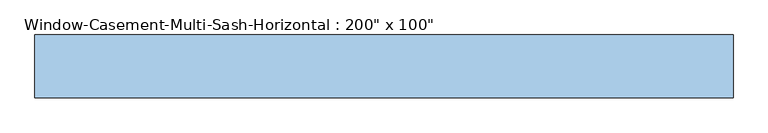
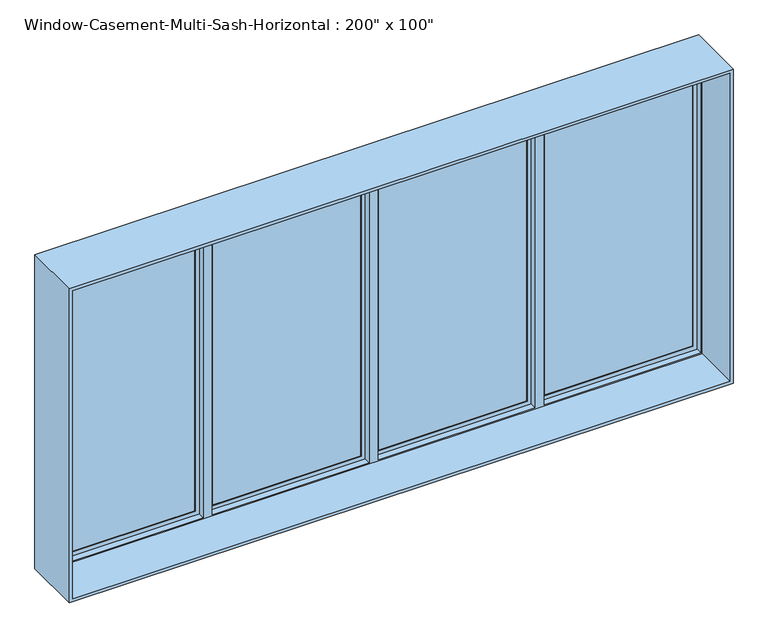
"""IFC4 building model written with IfcOpenShell, lengths in millimetres: window geometry."""

from ifc_helpers import new_model, si_unit, frame, origin, place, context, project, spatial, polyline, outline, extrude, faceted_brep, source, transform, mapped, element, save


def window_3db9eff8(model_context):
    return source(origin(), model_context, "Body", "SolidModel", [
        extrude(outline(polyline([(3429.0, 1295.4), (939.8, 1295.4), (939.8, 2514.6), (3429.0, 2514.6), (3429.0, 1295.4)]), holes=[polyline([(3387.1296875, 2472.7296875), (981.6703125, 2472.7296875), (981.6703125, 1337.2703125), (3387.1296875, 1337.2703125), (3387.1296875, 2472.7296875)])]), frame((0.0, 187.325, 0.0), z_axis=(0.0, 1.0, 0.0), x_axis=(0.0, 0.0, 1.0)), (0.0, 0.0, 1.0), 31.75),
        extrude(outline(polyline([(3429.0, -2514.6), (939.8, -2514.6), (939.8, -1295.4), (3429.0, -1295.4), (3429.0, -2514.6)]), holes=[polyline([(3387.1296875, -1337.2703125), (981.6703125, -1337.2703125), (981.6703125, -2472.7296875), (3387.1296875, -2472.7296875), (3387.1296875, -1337.2703125)])]), frame((0.0, 187.325, 0.0), z_axis=(0.0, 1.0, 0.0), x_axis=(0.0, 0.0, 1.0)), (0.0, 0.0, 1.0), 31.75),
        extrude(outline(polyline([(-1337.2703125, 212.725), (-1337.2703125, 206.375), (-2472.7296875, 206.375), (-2472.7296875, 212.725), (-1337.2703125, 212.725)])), frame((0.0, 0.0, 981.6703125), z_axis=(0.0, 0.0, 1.0), x_axis=(1.0, 0.0, 0.0)), (0.0, 0.0, 1.0), 2405.459375),
        extrude(outline(polyline([(-1337.2703125, 200.025), (-1337.2703125, 193.675), (-2472.7296875, 193.675), (-2472.7296875, 200.025), (-1337.2703125, 200.025)])), frame((0.0, 0.0, 981.6703125), z_axis=(0.0, 0.0, 1.0), x_axis=(1.0, 0.0, 0.0)), (0.0, 0.0, 1.0), 2405.459375),
        extrude(outline(polyline([(2472.7296875, 212.725), (2472.7296875, 206.375), (1337.2703125, 206.375), (1337.2703125, 212.725), (2472.7296875, 212.725)])), frame((0.0, 0.0, 981.6703125), z_axis=(0.0, 0.0, 1.0), x_axis=(1.0, 0.0, 0.0)), (0.0, 0.0, 1.0), 2405.459375),
        extrude(outline(polyline([(2472.7296875, 200.025), (2472.7296875, 193.675), (1337.2703125, 193.675), (1337.2703125, 200.025), (2472.7296875, 200.025)])), frame((0.0, 0.0, 981.6703125), z_axis=(0.0, 0.0, 1.0), x_axis=(1.0, 0.0, 0.0)), (0.0, 0.0, 1.0), 2405.459375),
        extrude(outline(polyline([(-67.2703125, 212.725), (-67.2703125, 206.375), (-1202.7296875, 206.375), (-1202.7296875, 212.725), (-67.2703125, 212.725)])), frame((0.0, 0.0, 981.6703125), z_axis=(0.0, 0.0, 1.0), x_axis=(1.0, 0.0, 0.0)), (0.0, 0.0, 1.0), 2405.459375),
        extrude(outline(polyline([(-67.2703125, 200.025), (-67.2703125, 193.675), (-1202.7296875, 193.675), (-1202.7296875, 200.025), (-67.2703125, 200.025)])), frame((0.0, 0.0, 981.6703125), z_axis=(0.0, 0.0, 1.0), x_axis=(1.0, 0.0, 0.0)), (0.0, 0.0, 1.0), 2405.459375),
        extrude(outline(polyline([(1202.7296875, 212.725), (1202.7296875, 206.375), (67.2703125, 206.375), (67.2703125, 212.725), (1202.7296875, 212.725)])), frame((0.0, 0.0, 981.6703125), z_axis=(0.0, 0.0, 1.0), x_axis=(1.0, 0.0, 0.0)), (0.0, 0.0, 1.0), 2405.459375),
        extrude(outline(polyline([(1202.7296875, 200.025), (1202.7296875, 193.675), (67.2703125, 193.675), (67.2703125, 200.025), (1202.7296875, 200.025)])), frame((0.0, 0.0, 981.6703125), z_axis=(0.0, 0.0, 1.0), x_axis=(1.0, 0.0, 0.0)), (0.0, 0.0, 1.0), 2405.459375),
        faceted_brep([(-1295.4, 187.325, 3429.0), (-2514.6, 187.325, 3429.0), (-2514.6, 228.6, 3429.0), (2514.6, 228.6, 3429.0), (2514.6, 187.325, 3429.0), (1295.4, 187.325, 3429.0), (1295.4, 225.425, 3429.0), (1244.6, 225.425, 3429.0), (1244.6, 187.325, 3429.0), (25.4, 187.325, 3429.0), (25.4, 225.425, 3429.0), (-25.4, 225.425, 3429.0), (-25.4, 187.325, 3429.0), (-1244.6, 187.325, 3429.0), (-1244.6, 225.425, 3429.0), (-1295.4, 225.425, 3429.0), (-2504.4796875, 136.525, 3418.8796875), (-2504.4796875, 187.325, 3418.8796875), (-1305.5203125, 187.325, 3418.8796875), (-1305.5203125, 136.525, 3418.8796875), (2504.4796875, 187.325, 3418.8796875), (2504.4796875, 136.525, 3418.8796875), (1305.5203125, 136.525, 3418.8796875), (1305.5203125, 187.325, 3418.8796875), (-1234.4796875, 187.325, 3418.8796875), (-35.5203125, 187.325, 3418.8796875), (-35.5203125, 136.525, 3418.8796875), (-1234.4796875, 136.525, 3418.8796875), (35.5203125, 187.325, 3418.8796875), (1234.4796875, 187.325, 3418.8796875), (1234.4796875, 136.525, 3418.8796875), (35.5203125, 136.525, 3418.8796875), (-2514.6, -228.6, 3429.0), (-2514.6, 136.525, 3429.0), (2514.6, 136.525, 3429.0), (2514.6, -228.6, 3429.0), (-2540.0, 228.6, 3454.4), (-2540.0, -228.6, 3454.4), (2540.0, -228.6, 3454.4), (2540.0, 228.6, 3454.4), (2514.6, 228.6, 939.8), (2514.6, 187.325, 939.8), (2504.4796875, 187.325, 949.9203125), (2504.4796875, 136.525, 949.9203125), (2514.6, 136.525, 939.8), (2514.6, -228.6, 939.8), (2540.0, -228.6, 914.4), (2540.0, 228.6, 914.4), (1295.4, 187.325, 939.8), (-2514.6, 228.6, 939.8), (-2514.6, 187.325, 939.8), (-1295.4, 187.325, 939.8), (-1295.4, 225.425, 939.8), (-1244.6, 225.425, 939.8), (-1244.6, 187.325, 939.8), (-25.4, 187.325, 939.8), (-25.4, 225.425, 939.8), (25.4, 225.425, 939.8), (25.4, 187.325, 939.8), (1244.6, 187.325, 939.8), (1244.6, 225.425, 939.8), (1295.4, 225.425, 939.8), (1305.5203125, 187.325, 949.9203125), (1305.5203125, 136.525, 949.9203125), (-2504.4796875, 187.325, 949.9203125), (-2504.4796875, 136.525, 949.9203125), (-1305.5203125, 136.525, 949.9203125), (-1305.5203125, 187.325, 949.9203125), (-35.5203125, 187.325, 949.9203125), (-1234.4796875, 187.325, 949.9203125), (-1234.4796875, 136.525, 949.9203125), (-35.5203125, 136.525, 949.9203125), (1234.4796875, 187.325, 949.9203125), (35.5203125, 187.325, 949.9203125), (35.5203125, 136.525, 949.9203125), (1234.4796875, 136.525, 949.9203125), (-2514.6, 136.525, 939.8), (-2514.6, -228.6, 939.8), (-2540.0, -228.6, 914.4), (-2540.0, 228.6, 914.4)], [[[0, 1, 2, 3, 4, 5, 6, 7, 8, 9, 10, 11, 12, 13, 14, 15]], [[16, 17, 18, 19]], [[20, 21, 22, 23]], [[24, 25, 26, 27]], [[28, 29, 30, 31]], [[32, 33, 34, 35]], [[36, 37, 38, 39]], [[4, 3, 40, 41]], [[21, 20, 42, 43]], [[35, 34, 44, 45]], [[39, 38, 46, 47]], [[48, 41, 40, 49, 50, 51, 52, 53, 54, 55, 56, 57, 58, 59, 60, 61]], [[43, 42, 62, 63]], [[64, 65, 66, 67]], [[68, 69, 70, 71]], [[72, 73, 74, 75]], [[45, 44, 76, 77]], [[47, 46, 78, 79]], [[2, 1, 50, 49]], [[4, 41, 48, 5], [20, 23, 62, 42]], [[50, 1, 0, 51], [64, 67, 18, 17]], [[12, 55, 54, 13], [69, 68, 25, 24]], [[8, 59, 58, 9], [73, 72, 29, 28]], [[17, 16, 65, 64]], [[44, 34, 33, 76], [16, 19, 66, 65], [27, 26, 71, 70], [31, 30, 75, 74], [21, 43, 63, 22]], [[33, 32, 77, 76]], [[38, 37, 78, 46], [32, 35, 45, 77]], [[37, 36, 79, 78]], [[36, 39, 47, 79], [3, 2, 49, 40]], [[18, 67, 66, 19]], [[69, 24, 27, 70]], [[53, 14, 13, 54]], [[14, 53, 52, 15]], [[15, 52, 51, 0]], [[25, 68, 71, 26]], [[73, 28, 31, 74]], [[57, 10, 9, 58]], [[10, 57, 56, 11]], [[11, 56, 55, 12]], [[6, 61, 60, 7]], [[7, 60, 59, 8]], [[29, 72, 75, 30]], [[62, 23, 22, 63]], [[61, 6, 5, 48]]]),
        extrude(outline(polyline([(3429.0, 25.4), (939.8, 25.4), (939.8, 1244.6), (3429.0, 1244.6), (3429.0, 25.4)]), holes=[polyline([(3387.1296875, 1202.7296875), (981.6703125, 1202.7296875), (981.6703125, 67.2703125), (3387.1296875, 67.2703125), (3387.1296875, 1202.7296875)])]), frame((0.0, 187.325, 0.0), z_axis=(0.0, 1.0, 0.0), x_axis=(0.0, 0.0, 1.0)), (0.0, 0.0, 1.0), 31.75),
        extrude(outline(polyline([(3429.0, -1244.6), (939.8, -1244.6), (939.8, -25.4), (3429.0, -25.4), (3429.0, -1244.6)]), holes=[polyline([(3387.1296875, -67.2703125), (981.6703125, -67.2703125), (981.6703125, -1202.7296875), (3387.1296875, -1202.7296875), (3387.1296875, -67.2703125)])]), frame((0.0, 187.325, 0.0), z_axis=(0.0, 1.0, 0.0), x_axis=(0.0, 0.0, 1.0)), (0.0, 0.0, 1.0), 31.75),
    ])


if __name__ == "__main__":
    model = new_model("IFC4")
    model_context = context("Model", 3, world=origin())
    ifc_project = project(units=[si_unit("LENGTHUNIT", "METRE", prefix="MILLI")], contexts=[model_context])
    site = spatial("IfcSite", under=ifc_project)
    building = spatial("IfcBuilding", under=site)
    placement = place(None, origin())
    window_shape = window_3db9eff8(model_context)
    element("IfcWindow", 1, ObjectType="Window-Casement-Multi-Sash-Horizontal : 200\" x 100\"", at=placement, inside=building, context=model_context, shape_type="MappedRepresentation", body=[
        mapped(window_shape, transform((0.0, 0.0, 0.0), x_axis=(1.0, 0.0, 0.0), y_axis=(0.0, 1.0, 0.0), z_axis=(0.0, 0.0, 1.0))),
    ])
    save(model, "model.ifc")

# Revit data of these elements
# Type "Window-Casement-Multi-Sash-Horizontal : 200\" x 100\""
#   Type Mark = "50"
#   Fire Rating = "0.5h"
#   Assembly Code = "B2020100"
#   Analytic Construction = "Double glazing - domestic"
#   Window Inset [instance default] = 0' - 0 5/8"
#   Wall Thickness [instance default] = 0' - 6"
#   Visual Light Transmittance = 0.81
#   Thermal Resistance (R) = 0.319569 (m²·K)/W
#   Solar Heat Gain Coefficient = 0.76
#   Rough Width = 16' - 8 1/2"
#   Rough Height = 8' - 4 1/2"
#   Open Window Width = 4' - 2"
#   Heat Transfer Coefficient (U) = 3.12929 W/(m²·K)
#   Height = 8' - 4"
#   Frame Gap 3 [instance default] = 0' - 1 83/128"
#   Frame Gap 2 [instance default] = 0' - 0 5/8"
#   Frame Gap 1 = 0' - 1 51/128"
#   Default Sill Height = 3' - 0"
#   Width = 16' - 8"
#   Frame Material = Metal - Aluminum
#   Glass Panel Material = Glass
#   Wall Closure = (empty or 0)
# Element 1 (IfcWindow, "Window-Casement-Multi-Sash-Horizontal : 200\" x 100\"")
#   Wall Thickness = 1' - 6"
#   Materials on its faces: "Metal - Aluminum", "Glass"
# Materials
#   "Metal - Aluminum": class "Metal", colour RGB 247 247 247, transparency 0
#   "Glass": class "Glass", colour RGB 0 128 192, transparency 0.9, Description = "Soda Lime Glass", Cost = 0
